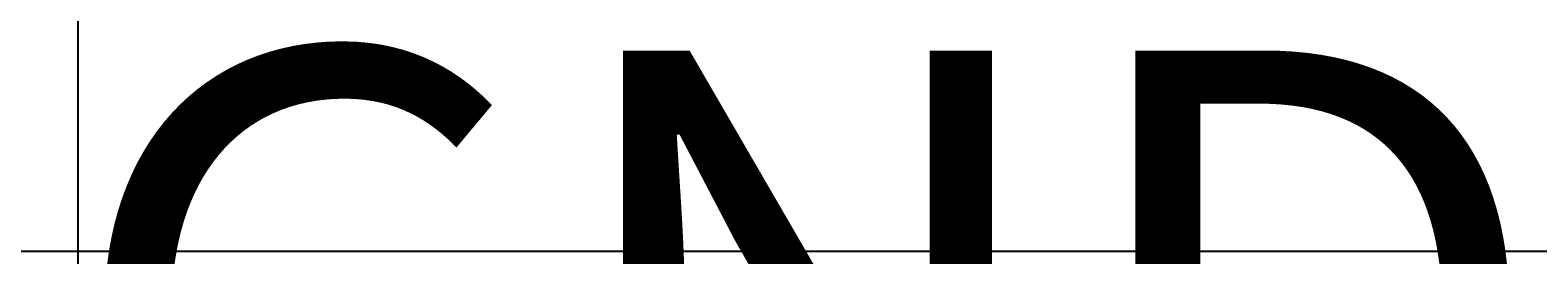
# Model space of a CAD drawing. Units: inches. Extents: x 35362 to 73946, y 43607 to 67532.
# Tile 97 of 134: x 50119 to 50761, y 48969 to 49064. Entities that reach past the tile are written whole.
import ezdxf

# ---------------------------------------------------------------- set-up
doc = ezdxf.new("R2010")
doc.units = ezdxf.units.IN
doc.header["$MEASUREMENT"] = 0
doc.layers.add('A-ANNO-DIMS', color=2, linetype='Continuous', lineweight=18)
doc.layers.add('E-ANNO-TEXT', color=5, linetype='Continuous', lineweight=18)
doc.styles.get("Standard").update_dxf_attribs({"font": 'arial.ttf'})
doc.dimstyles.get("Standard").update_dxf_attribs({"dimtxt": 0.18, "dimasz": 0.18, "dimexe": 0.18, "dimexo": 0.0625, "dimgap": 0.09, "dimtad": 0, "dimtih": 1, "dimtoh": 1, "dimdec": 4, "dimzin": 0, "dimdsep": 46, "dimtxsty": 'Standard', "dimcen": 0.09, "dimadec": 0, "dimazin": 0, "dimtfac": 1, "dimtdec": 4, "dimtofl": 0, "dimtmove": 0, "dimatfit": 3, "dimfxl": 1, "dimtolj": 1, "dimtzin": 0, "dimarcsym": 0})

# ---------------------------------------------------------------- blocks, each defined once
blk = doc.blocks.new('*D11')
at = {"layer": 'A-ANNO-DIMS', "color": 0, "lineweight": -2, "transparency": 16777216}
for p, q in [((47978.66, 56028.77), (47978.66, 43606.68)), ((53109.76, 56028.77), (53109.76, 43606.68)), ((47978.84, 43606.86), (50543.87, 43606.86)), ((53109.58, 43606.86), (50544.55, 43606.86))]:
    blk.add_line(p, q, dxfattribs=at)
at = {"layer": 'A-ANNO-DIMS', "color": 0, "transparency": 16777216}
for points in [[(47978.84, 43606.89), (47978.84, 43606.83), (47978.66, 43606.86)], [(53109.58, 43606.89), (53109.58, 43606.83), (53109.76, 43606.86)]]:
    blk.add_solid(points, dxfattribs=at)
at = {"layer": 'Defpoints', "color": 0, "transparency": 16777216}
for p in [(47978.66, 56028.84), (53109.76, 56028.84), (53109.76, 43606.86)]:
    blk.add_point(p, dxfattribs=at)
at = {"layer": 'A-ANNO-DIMS', "color": 0, "transparency": 16777216, "insert": (50544.21, 43606.86), "char_height": 0.18, "attachment_point": 5}
blk.add_mtext('\\A1;5131', dxfattribs=at)
blk = doc.blocks.new('*D13')
at = {"layer": 'A-ANNO-DIMS', "color": 0, "lineweight": -2, "transparency": 16777216}
for p, q in [((48373.49, 51694.02), (48373.49, 43606.68)), ((51029.04, 51694.02), (51029.04, 43606.68)), ((48373.67, 43606.86), (49700.8, 43606.86)), ((51028.86, 43606.86), (49701.73, 43606.86))]:
    blk.add_line(p, q, dxfattribs=at)
at = {"layer": 'A-ANNO-DIMS', "color": 0, "transparency": 16777216}
for points in [[(48373.67, 43606.89), (48373.67, 43606.83), (48373.49, 43606.86)], [(51028.86, 43606.89), (51028.86, 43606.83), (51029.04, 43606.86)]]:
    blk.add_solid(points, dxfattribs=at)
at = {"layer": 'Defpoints', "color": 0, "transparency": 16777216}
for p in [(48373.49, 51694.09), (51029.04, 51694.09), (51029.04, 43606.86)]:
    blk.add_point(p, dxfattribs=at)
at = {"layer": 'A-ANNO-DIMS', "color": 0, "transparency": 16777216, "insert": (49701.27, 43606.86), "char_height": 0.18, "attachment_point": 5}
blk.add_mtext('\\A1;2655.6', dxfattribs=at)
blk = doc.blocks.new('*D17')
at = {"layer": 'A-ANNO-DIMS', "color": 0, "lineweight": -2, "transparency": 16777216}
for p, q in [((49923.31, 61293.22), (49923.31, 43606.68)), ((51913.93, 61293.22), (51913.93, 43606.68)), ((49923.49, 43606.86), (50918.16, 43606.86)), ((51913.75, 43606.86), (50919.07, 43606.86))]:
    blk.add_line(p, q, dxfattribs=at)
at = {"layer": 'A-ANNO-DIMS', "color": 0, "transparency": 16777216}
for points in [[(49923.49, 43606.89), (49923.49, 43606.83), (49923.31, 43606.86)], [(51913.75, 43606.89), (51913.75, 43606.83), (51913.93, 43606.86)]]:
    blk.add_solid(points, dxfattribs=at)
at = {"layer": 'Defpoints', "color": 0, "transparency": 16777216}
for p in [(49923.31, 61293.29), (51913.93, 61293.29), (51913.93, 43606.86)]:
    blk.add_point(p, dxfattribs=at)
at = {"layer": 'A-ANNO-DIMS', "color": 0, "transparency": 16777216, "insert": (50918.62, 43606.86), "char_height": 0.18, "attachment_point": 5}
blk.add_mtext('\\A1;1990.6', dxfattribs=at)
blk = doc.blocks.new('*D67')
at = {"layer": 'A-ANNO-DIMS', "color": 0, "lineweight": -2, "transparency": 16777216}
for p, q in [((56873.54, 53351.53), (35361.77, 53351.53)), ((35361.95, 53351.35), (35361.95, 49400.89)), ((35361.95, 45450.07), (35361.95, 49400.53)), ((53793.58, 45449.89), (35361.77, 45449.89))]:
    blk.add_line(p, q, dxfattribs=at)
at = {"layer": 'A-ANNO-DIMS', "color": 0, "transparency": 16777216}
for points in [[(35361.92, 53351.35), (35361.98, 53351.35), (35361.95, 53351.53)], [(35361.92, 45450.07), (35361.98, 45450.07), (35361.95, 45449.89)]]:
    blk.add_solid(points, dxfattribs=at)
at = {"layer": 'Defpoints', "color": 0, "transparency": 16777216}
for p in [(35361.95, 53351.53), (56873.6, 53351.53), (53793.64, 45449.89)]:
    blk.add_point(p, dxfattribs=at)
at = {"layer": 'A-ANNO-DIMS', "color": 0, "transparency": 16777216, "insert": (35361.95, 49400.71), "char_height": 0.18, "attachment_point": 5}
blk.add_mtext('\\A1;7901.6', dxfattribs=at)
blk = doc.blocks.new('*D84')
at = {"layer": 'A-ANNO-DIMS', "color": 0, "lineweight": -2, "transparency": 16777216}
for p, q in [((55540.23, 49259.94), (35361.77, 49259.94)), ((35361.95, 49259.76), (35361.95, 49115.14)), ((35361.95, 48970.16), (35361.95, 49114.78)), ((55540.23, 48969.98), (35361.77, 48969.98))]:
    blk.add_line(p, q, dxfattribs=at)
at = {"layer": 'A-ANNO-DIMS', "color": 0, "transparency": 16777216}
for points in [[(35361.92, 49259.76), (35361.98, 49259.76), (35361.95, 49259.94)], [(35361.92, 48970.16), (35361.98, 48970.16), (35361.95, 48969.98)]]:
    blk.add_solid(points, dxfattribs=at)
at = {"layer": 'Defpoints', "color": 0, "transparency": 16777216}
for p in [(35361.95, 49259.94), (55540.3, 49259.94), (55540.3, 48969.98)]:
    blk.add_point(p, dxfattribs=at)
at = {"layer": 'A-ANNO-DIMS', "color": 0, "transparency": 16777216, "insert": (35361.95, 49114.96), "char_height": 0.18, "attachment_point": 5}
blk.add_mtext('\\A1;289.96', dxfattribs=at)
blk = doc.blocks.new('*D86')
at = {"layer": 'A-ANNO-DIMS', "color": 0, "lineweight": -2, "transparency": 16777216}
for p, q in [((51285.53, 49320.08), (35361.77, 49320.08)), ((35361.95, 49319.9), (35361.95, 49120.26)), ((35361.95, 48920.26), (35361.95, 49119.9)), ((51285.53, 48920.08), (35361.77, 48920.08))]:
    blk.add_line(p, q, dxfattribs=at)
at = {"layer": 'A-ANNO-DIMS', "color": 0, "transparency": 16777216}
for points in [[(35361.92, 49319.9), (35361.98, 49319.9), (35361.95, 49320.08)], [(35361.92, 48920.26), (35361.98, 48920.26), (35361.95, 48920.08)]]:
    blk.add_solid(points, dxfattribs=at)
at = {"layer": 'Defpoints', "color": 0, "transparency": 16777216}
for p in [(35361.95, 49320.08), (51285.59, 49320.08), (51285.59, 48920.08)]:
    blk.add_point(p, dxfattribs=at)
at = {"layer": 'A-ANNO-DIMS', "color": 0, "transparency": 16777216, "insert": (35361.95, 49120.08), "char_height": 0.18, "attachment_point": 5}
blk.add_mtext('\\A1;400.0', dxfattribs=at)
blk = doc.blocks.new('*D107')
at = {"layer": 'A-ANNO-DIMS', "color": 0, "lineweight": -2, "transparency": 16777216}
for p, q in [((50139.56, 59850.01), (50139.56, 43606.68)), ((51320.81, 59850.01), (51320.81, 43606.68)), ((50139.74, 43606.86), (50729.73, 43606.86)), ((51320.63, 43606.86), (50730.64, 43606.86))]:
    blk.add_line(p, q, dxfattribs=at)
at = {"layer": 'A-ANNO-DIMS', "color": 0, "transparency": 16777216}
for points in [[(50139.74, 43606.89), (50139.74, 43606.83), (50139.56, 43606.86)], [(51320.63, 43606.89), (51320.63, 43606.83), (51320.81, 43606.86)]]:
    blk.add_solid(points, dxfattribs=at)
at = {"layer": 'Defpoints', "color": 0, "transparency": 16777216}
for p in [(50139.56, 59850.08), (51320.81, 59850.08), (51320.81, 43606.86)]:
    blk.add_point(p, dxfattribs=at)
at = {"layer": 'A-ANNO-DIMS', "color": 0, "transparency": 16777216, "insert": (50730.19, 43606.86), "char_height": 0.18, "attachment_point": 5}
blk.add_mtext('\\A1;1181.3', dxfattribs=at)

msp = doc.modelspace()

# ---------------------------------------------------------------- texts
at = {"layer": 'E-ANNO-TEXT'}
msp.add_text('GND', height=220.866, dxfattribs=at).set_placement((50133.331, 48834.598))

# ---------------------------------------------------------------- dimensions: what is measured, and where the dimension line sits
at = {"layer": 'A-ANNO-DIMS'}
for base, p1, p2, override, picture, middle in [((51913.931, 43606.859), (49923.307, 61293.286), (51913.931, 61293.286), {"dimdec": 1, "dimlfac": 1, "dimrnd": 0, "dimzin": 0, "dimdsep": 46, "dimlunit": 2}, '*D17', (50918.619, 43606.859)), ((51320.8133, 43606.859), (50139.5627, 59850.0769), (51320.8133, 59850.0769), {"dimdec": 1, "dimlfac": 1, "dimrnd": 0, "dimzin": 0, "dimdsep": 46, "dimlunit": 2}, '*D107', (50730.188, 43606.859)), ((53109.76, 43606.859), (47978.665, 56028.836), (53109.76, 56028.836), {"dimdec": 0, "dimlfac": 1, "dimrnd": 0, "dimzin": 0, "dimdsep": 46, "dimlunit": 2}, '*D11', (50544.212, 43606.859)), ((51029.043, 43606.859), (48373.492, 51694.087), (51029.043, 51694.087), {"dimdec": 1, "dimlfac": 1, "dimrnd": 0, "dimzin": 0, "dimdsep": 46, "dimlunit": 2}, '*D13', (49701.267, 43606.859))]:
    dim = msp.add_linear_dim(base=base, p1=p1, p2=p2, dimstyle='Standard', override=override, dxfattribs=at)
    dim.commit()
    dim.dimension.update_dxf_attribs({"geometry": picture, "text_midpoint": middle})
for base, p1, p2, override, picture, middle in [((35361.949, 53351.529), (53793.638, 45449.894), (56873.602, 53351.529), {"dimdec": 1, "dimlfac": 1, "dimrnd": 0, "dimzin": 0, "dimdsep": 46, "dimlunit": 2}, '*D67', (35361.949, 49400.712)), ((35361.949, 49320.079), (51285.595, 48920.079), (51285.595, 49320.079), {"dimdec": 1, "dimlfac": 1, "dimrnd": 0, "dimzin": 0, "dimdsep": 46, "dimlunit": 2}, '*D86', (35361.949, 49120.079)), ((35361.9491, 49259.9353), (55540.2972, 48969.9796), (55540.2972, 49259.9353), {"dimdec": 2, "dimlfac": 1, "dimrnd": 0, "dimzin": 0, "dimdsep": 46, "dimlunit": 2}, '*D84', (35361.9491, 49114.9575))]:
    dim = msp.add_linear_dim(base=base, p1=p1, p2=p2, angle=90, dimstyle='Standard', override=override, dxfattribs=at)
    dim.commit()
    dim.dimension.update_dxf_attribs({"geometry": picture, "text_midpoint": middle})

doc.saveas('drawing.dxf')
